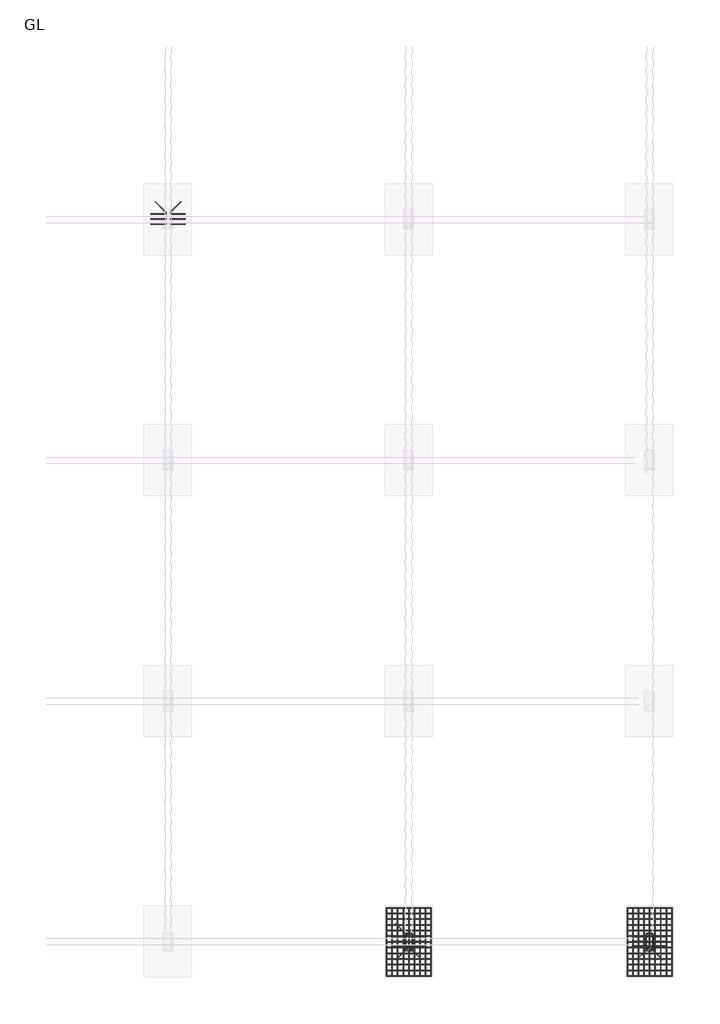
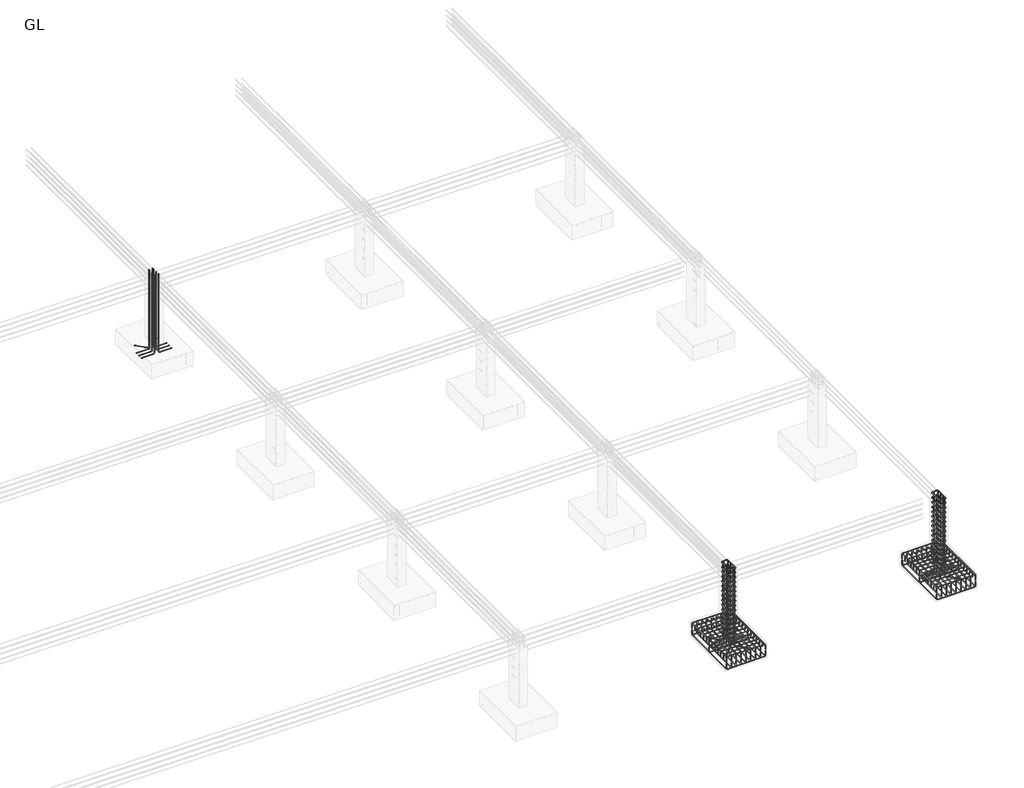
# One storey, part 10 of 16: 23 reinforcing bars.
"""IFC4 building model written with IfcOpenShell, lengths in millimetres."""

from ifc_helpers import new_model, si_unit, point, frame, origin, place, context, project, spatial, polyline, circle_curve, trimmed, segment, composite_curve, source, transform, mapped, element, save
from ifc_brep_helpers import swept_disk

model = new_model("IFC4")

# Units and contexts
model_context = context("Model", 3, world=origin())
ifc_project = project(units=[si_unit("LENGTHUNIT", "METRE", prefix="MILLI")], contexts=[model_context])

# Site, building, storey
site = spatial("IfcSite", under=ifc_project)
building = spatial("IfcBuilding", under=site)
storey = spatial("IfcBuildingStorey", under=building, Name="GL", Elevation=-1829.0)

# Reinforcing bars
placement = place(None, origin())
reinforcing_bar_shape = source(origin(), model_context, "Body", "SolidModel", [
    swept_disk(composite_curve([segment(polyline([(2141.0455621, -19415.1167521, -2089.0), (2141.0455621, -19415.1167521, -2213.0)]), True, "CONTINUOUS"), segment(trimmed(circle_curve(frame((2111.0455621, -19415.1167521, -2213.0), z_axis=(0.0, 1.0, 0.0), x_axis=(30.0, 0.0, 0.0)), 30.0), [point((2141.0455621, -19415.1167521, -2213.0))], [point((2111.0455621, -19415.1167521, -2243.0))], True, "CARTESIAN"), True, "CONTINUOUS"), segment(polyline([(2111.0455621, -19415.1167521, -2243.0), (1043.0455621, -19415.1167521, -2243.0)]), True, "CONTINUOUS"), segment(trimmed(circle_curve(frame((1043.0455621, -19415.1167521, -2213.0), z_axis=(0.0, 1.0, 0.0), x_axis=(0.0, 0.0, -30.0)), 30.0), [point((1043.0455621, -19415.1167521, -2243.0))], [point((1013.0455621, -19415.1167521, -2213.0))], True, "CARTESIAN"), True, "CONTINUOUS"), segment(polyline([(1013.0455621, -19415.1167521, -2213.0), (1013.0455621, -19415.1167521, -2089.0)]), True, "CONTINUOUS")], self_intersect=False), 6.0),
])
element("IfcReinforcingBar", 1, at=placement, inside=storey, context=model_context, shape_type="MappedRepresentation", body=[
    mapped(reinforcing_bar_shape, transform((0.0, 0.0, 0.0), x_axis=(1.0, 0.0, 0.0), y_axis=(0.0, 1.0, 0.0), z_axis=(0.0, 0.0, 1.0))),
    mapped(reinforcing_bar_shape, transform((0.0, -864.0, 0.0), x_axis=(1.0, 0.0, 0.0), y_axis=(0.0, 1.0, 0.0), z_axis=(0.0, 0.0, 1.0))),
    mapped(reinforcing_bar_shape, transform((0.0, -1728.0, 0.0), x_axis=(1.0, 0.0, 0.0), y_axis=(0.0, 1.0, 0.0), z_axis=(0.0, 0.0, 1.0))),
])
reinforcing_bar_2_shape = source(origin(), model_context, "Body", "SolidModel", [
    swept_disk(composite_curve([segment(polyline([(1013.0455621, -19415.1167521, -2022.436678), (1013.0455621, -19415.1167521, -1898.436678)]), True, "CONTINUOUS"), segment(trimmed(circle_curve(frame((1043.0455621, -19415.1167521, -1898.436678), z_axis=(0.0, 1.0, 0.0), x_axis=(-30.000000000000114, 0.0, 0.0)), 30.0), [point((1013.0455621, -19415.1167521, -1898.436678))], [point((1043.0455621, -19415.1167521, -1868.436678))], True, "CARTESIAN"), True, "CONTINUOUS"), segment(polyline([(1043.0455621, -19415.1167521, -1868.436678), (2111.0455621, -19415.1167521, -1868.436678)]), True, "CONTINUOUS"), segment(trimmed(circle_curve(frame((2111.0455621, -19415.1167521, -1898.436678), z_axis=(0.0, 1.0, 0.0), x_axis=(0.0, 0.0, 30.0)), 30.0), [point((2111.0455621, -19415.1167521, -1868.436678))], [point((2141.0455621, -19415.1167521, -1898.436678))], True, "CARTESIAN"), True, "CONTINUOUS"), segment(polyline([(2141.0455621, -19415.1167521, -1898.436678), (2141.0455621, -19415.1167521, -2022.436678)]), True, "CONTINUOUS")], self_intersect=False), 6.0),
])
element("IfcReinforcingBar", 2, at=placement, inside=storey, context=model_context, shape_type="MappedRepresentation", body=[
    mapped(reinforcing_bar_2_shape, transform((0.0, 0.0, 0.0), x_axis=(1.0, 0.0, 0.0), y_axis=(0.0, 1.0, 0.0), z_axis=(0.0, 0.0, 1.0))),
    mapped(reinforcing_bar_2_shape, transform((0.0, -144.0, 0.0), x_axis=(1.0, 0.0, 0.0), y_axis=(0.0, 1.0, 0.0), z_axis=(0.0, 0.0, 1.0))),
    mapped(reinforcing_bar_2_shape, transform((0.0, -288.0, 0.0), x_axis=(1.0, 0.0, 0.0), y_axis=(0.0, 1.0, 0.0), z_axis=(0.0, 0.0, 1.0))),
    mapped(reinforcing_bar_2_shape, transform((0.0, -432.0, 0.0), x_axis=(1.0, 0.0, 0.0), y_axis=(0.0, 1.0, 0.0), z_axis=(0.0, 0.0, 1.0))),
    mapped(reinforcing_bar_2_shape, transform((0.0, -576.0, 0.0), x_axis=(1.0, 0.0, 0.0), y_axis=(0.0, 1.0, 0.0), z_axis=(0.0, 0.0, 1.0))),
    mapped(reinforcing_bar_2_shape, transform((0.0, -720.0, 0.0), x_axis=(1.0, 0.0, 0.0), y_axis=(0.0, 1.0, 0.0), z_axis=(0.0, 0.0, 1.0))),
    mapped(reinforcing_bar_2_shape, transform((0.0, -864.0, 0.0), x_axis=(1.0, 0.0, 0.0), y_axis=(0.0, 1.0, 0.0), z_axis=(0.0, 0.0, 1.0))),
    mapped(reinforcing_bar_2_shape, transform((0.0, -1008.0, 0.0), x_axis=(1.0, 0.0, 0.0), y_axis=(0.0, 1.0, 0.0), z_axis=(0.0, 0.0, 1.0))),
    mapped(reinforcing_bar_2_shape, transform((0.0, -1152.0, 0.0), x_axis=(1.0, 0.0, 0.0), y_axis=(0.0, 1.0, 0.0), z_axis=(0.0, 0.0, 1.0))),
    mapped(reinforcing_bar_2_shape, transform((0.0, -1296.0, 0.0), x_axis=(1.0, 0.0, 0.0), y_axis=(0.0, 1.0, 0.0), z_axis=(0.0, 0.0, 1.0))),
    mapped(reinforcing_bar_2_shape, transform((0.0, -1440.0, 0.0), x_axis=(1.0, 0.0, 0.0), y_axis=(0.0, 1.0, 0.0), z_axis=(0.0, 0.0, 1.0))),
    mapped(reinforcing_bar_2_shape, transform((0.0, -1584.0, 0.0), x_axis=(1.0, 0.0, 0.0), y_axis=(0.0, 1.0, 0.0), z_axis=(0.0, 0.0, 1.0))),
    mapped(reinforcing_bar_2_shape, transform((0.0, -1728.0, 0.0), x_axis=(1.0, 0.0, 0.0), y_axis=(0.0, 1.0, 0.0), z_axis=(0.0, 0.0, 1.0))),
])
reinforcing_bar_3_shape = source(origin(), model_context, "Body", "SolidModel", [
    swept_disk(composite_curve([segment(polyline([(1013.0455621, -21143.1167521, -2027.5081232), (1013.0455621, -21143.1167521, -1903.5081232)]), True, "CONTINUOUS"), segment(trimmed(circle_curve(frame((1013.0455621, -21113.1167521, -1903.5081232), z_axis=(-1.0, 0.0, 0.0), x_axis=(0.0, -30.0, 0.0)), 30.0), [point((1013.0455621, -21143.1167521, -1903.5081232))], [point((1013.0455621, -21113.1167521, -1873.5081232))], True, "CARTESIAN"), True, "CONTINUOUS"), segment(polyline([(1013.0455621, -21113.1167521, -1873.5081232), (1013.0455621, -19445.1167521, -1873.5081232)]), True, "CONTINUOUS"), segment(trimmed(circle_curve(frame((1013.0455621, -19445.1167521, -1903.5081232), z_axis=(-1.0, 0.0, 0.0), x_axis=(0.0, 0.0, 30.0)), 30.0), [point((1013.0455621, -19445.1167521, -1873.5081232))], [point((1013.0455621, -19415.1167521, -1903.5081232))], True, "CARTESIAN"), True, "CONTINUOUS"), segment(polyline([(1013.0455621, -19415.1167521, -1903.5081232), (1013.0455621, -19415.1167521, -2027.5081232)]), True, "CONTINUOUS")], self_intersect=False), 6.0),
])
element("IfcReinforcingBar", 3, at=placement, inside=storey, context=model_context, shape_type="MappedRepresentation", body=[
    mapped(reinforcing_bar_3_shape, transform((0.0, 0.0, 0.0), x_axis=(1.0, 0.0, 0.0), y_axis=(0.0, 1.0, 0.0), z_axis=(0.0, 0.0, 1.0))),
    mapped(reinforcing_bar_3_shape, transform((141.0, 0.0, 0.0), x_axis=(1.0, 0.0, 0.0), y_axis=(0.0, 1.0, 0.0), z_axis=(0.0, 0.0, 1.0))),
    mapped(reinforcing_bar_3_shape, transform((282.0, 0.0, 0.0), x_axis=(1.0, 0.0, 0.0), y_axis=(0.0, 1.0, 0.0), z_axis=(0.0, 0.0, 1.0))),
    mapped(reinforcing_bar_3_shape, transform((423.0, 0.0, 0.0), x_axis=(1.0, 0.0, 0.0), y_axis=(0.0, 1.0, 0.0), z_axis=(0.0, 0.0, 1.0))),
    mapped(reinforcing_bar_3_shape, transform((564.0, 0.0, 0.0), x_axis=(1.0, 0.0, 0.0), y_axis=(0.0, 1.0, 0.0), z_axis=(0.0, 0.0, 1.0))),
    mapped(reinforcing_bar_3_shape, transform((705.0, 0.0, 0.0), x_axis=(1.0, 0.0, 0.0), y_axis=(0.0, 1.0, 0.0), z_axis=(0.0, 0.0, 1.0))),
    mapped(reinforcing_bar_3_shape, transform((846.0, 0.0, 0.0), x_axis=(1.0, 0.0, 0.0), y_axis=(0.0, 1.0, 0.0), z_axis=(0.0, 0.0, 1.0))),
    mapped(reinforcing_bar_3_shape, transform((987.0, 0.0, 0.0), x_axis=(1.0, 0.0, 0.0), y_axis=(0.0, 1.0, 0.0), z_axis=(0.0, 0.0, 1.0))),
    mapped(reinforcing_bar_3_shape, transform((1128.0, 0.0, 0.0), x_axis=(1.0, 0.0, 0.0), y_axis=(0.0, 1.0, 0.0), z_axis=(0.0, 0.0, 1.0))),
])
reinforcing_bar_4_shape = source(origin(), model_context, "Body", "SolidModel", [
    swept_disk(composite_curve([segment(polyline([(2141.0455621, -21143.1167521, -2080.6239909), (2141.0455621, -21143.1167521, -2204.6239909)]), True, "CONTINUOUS"), segment(trimmed(circle_curve(frame((2141.0455621, -21113.1167521, -2204.6239909), z_axis=(1.0, 0.0, 0.0), x_axis=(0.0, -30.0, 0.0)), 30.0), [point((2141.0455621, -21143.1167521, -2204.6239909))], [point((2141.0455621, -21113.1167521, -2234.6239909))], True, "CARTESIAN"), True, "CONTINUOUS"), segment(polyline([(2141.0455621, -21113.1167521, -2234.6239909), (2141.0455621, -19458.1421892, -2234.6239909)]), True, "CONTINUOUS"), segment(trimmed(circle_curve(frame((2141.0455621, -19458.1421892, -2204.6239909), z_axis=(1.0, 0.0, 0.0), x_axis=(0.0, 0.0, -30.0)), 30.0), [point((2141.0455621, -19458.1421892, -2234.6239909))], [point((2141.0455621, -19428.1421892, -2204.6239909))], True, "CARTESIAN"), True, "CONTINUOUS"), segment(polyline([(2141.0455621, -19428.1421892, -2204.6239909), (2141.0455621, -19428.1421892, -2080.6239909)]), True, "CONTINUOUS")], self_intersect=False), 6.0),
])
element("IfcReinforcingBar", 4, at=placement, inside=storey, context=model_context, shape_type="MappedRepresentation", body=[
    mapped(reinforcing_bar_4_shape, transform((0.0, 0.0, 0.0), x_axis=(1.0, 0.0, 0.0), y_axis=(0.0, 1.0, 0.0), z_axis=(0.0, 0.0, 1.0))),
    mapped(reinforcing_bar_4_shape, transform((-141.0, 0.0, 0.0), x_axis=(1.0, 0.0, 0.0), y_axis=(0.0, 1.0, 0.0), z_axis=(0.0, 0.0, 1.0))),
    mapped(reinforcing_bar_4_shape, transform((-282.0, 0.0, 0.0), x_axis=(1.0, 0.0, 0.0), y_axis=(0.0, 1.0, 0.0), z_axis=(0.0, 0.0, 1.0))),
    mapped(reinforcing_bar_4_shape, transform((-423.0, 0.0, 0.0), x_axis=(1.0, 0.0, 0.0), y_axis=(0.0, 1.0, 0.0), z_axis=(0.0, 0.0, 1.0))),
    mapped(reinforcing_bar_4_shape, transform((-564.0, 0.0, 0.0), x_axis=(1.0, 0.0, 0.0), y_axis=(0.0, 1.0, 0.0), z_axis=(0.0, 0.0, 1.0))),
    mapped(reinforcing_bar_4_shape, transform((-705.0, 0.0, 0.0), x_axis=(1.0, 0.0, 0.0), y_axis=(0.0, 1.0, 0.0), z_axis=(0.0, 0.0, 1.0))),
    mapped(reinforcing_bar_4_shape, transform((-846.0, 0.0, 0.0), x_axis=(1.0, 0.0, 0.0), y_axis=(0.0, 1.0, 0.0), z_axis=(0.0, 0.0, 1.0))),
    mapped(reinforcing_bar_4_shape, transform((-987.0, 0.0, 0.0), x_axis=(1.0, 0.0, 0.0), y_axis=(0.0, 1.0, 0.0), z_axis=(0.0, 0.0, 1.0))),
    mapped(reinforcing_bar_4_shape, transform((-1128.0, 0.0, 0.0), x_axis=(1.0, 0.0, 0.0), y_axis=(0.0, 1.0, 0.0), z_axis=(0.0, 0.0, 1.0))),
])
reinforcing_bar_5_shape = source(origin(), model_context, "Body", "SolidModel", [
    swept_disk(composite_curve([segment(polyline([(8237.0455621, -19415.1167521, -2089.0), (8237.0455621, -19415.1167521, -2213.0)]), True, "CONTINUOUS"), segment(trimmed(circle_curve(frame((8207.0455621, -19415.1167521, -2213.0), z_axis=(0.0, 1.0, 0.0), x_axis=(30.0, 0.0, 0.0)), 30.0), [point((8237.0455621, -19415.1167521, -2213.0))], [point((8207.0455621, -19415.1167521, -2243.0))], True, "CARTESIAN"), True, "CONTINUOUS"), segment(polyline([(8207.0455621, -19415.1167521, -2243.0), (7139.0455621, -19415.1167521, -2243.0)]), True, "CONTINUOUS"), segment(trimmed(circle_curve(frame((7139.0455621, -19415.1167521, -2213.0), z_axis=(0.0, 1.0, 0.0), x_axis=(0.0, 0.0, -30.0)), 30.0), [point((7139.0455621, -19415.1167521, -2243.0))], [point((7109.0455621, -19415.1167521, -2213.0))], True, "CARTESIAN"), True, "CONTINUOUS"), segment(polyline([(7109.0455621, -19415.1167521, -2213.0), (7109.0455621, -19415.1167521, -2089.0)]), True, "CONTINUOUS")], self_intersect=False), 6.0),
])
element("IfcReinforcingBar", 5, at=placement, inside=storey, context=model_context, shape_type="MappedRepresentation", body=[
    mapped(reinforcing_bar_5_shape, transform((0.0, 0.0, 0.0), x_axis=(1.0, 0.0, 0.0), y_axis=(0.0, 1.0, 0.0), z_axis=(0.0, 0.0, 1.0))),
    mapped(reinforcing_bar_5_shape, transform((0.0, -864.0, 0.0), x_axis=(1.0, 0.0, 0.0), y_axis=(0.0, 1.0, 0.0), z_axis=(0.0, 0.0, 1.0))),
    mapped(reinforcing_bar_5_shape, transform((0.0, -1728.0, 0.0), x_axis=(1.0, 0.0, 0.0), y_axis=(0.0, 1.0, 0.0), z_axis=(0.0, 0.0, 1.0))),
])
reinforcing_bar_6_shape = source(origin(), model_context, "Body", "SolidModel", [
    swept_disk(composite_curve([segment(polyline([(7109.0455621, -19415.1167521, -2022.436678), (7109.0455621, -19415.1167521, -1898.436678)]), True, "CONTINUOUS"), segment(trimmed(circle_curve(frame((7139.0455621, -19415.1167521, -1898.436678), z_axis=(0.0, 1.0, 0.0), x_axis=(-30.0, 0.0, 0.0)), 30.0), [point((7109.0455621, -19415.1167521, -1898.436678))], [point((7139.0455621, -19415.1167521, -1868.436678))], True, "CARTESIAN"), True, "CONTINUOUS"), segment(polyline([(7139.0455621, -19415.1167521, -1868.436678), (8207.0455621, -19415.1167521, -1868.436678)]), True, "CONTINUOUS"), segment(trimmed(circle_curve(frame((8207.0455621, -19415.1167521, -1898.436678), z_axis=(0.0, 1.0, 0.0), x_axis=(0.0, 0.0, 30.0)), 30.0), [point((8207.0455621, -19415.1167521, -1868.436678))], [point((8237.0455621, -19415.1167521, -1898.436678))], True, "CARTESIAN"), True, "CONTINUOUS"), segment(polyline([(8237.0455621, -19415.1167521, -1898.436678), (8237.0455621, -19415.1167521, -2022.436678)]), True, "CONTINUOUS")], self_intersect=False), 6.0),
])
element("IfcReinforcingBar", 6, at=placement, inside=storey, context=model_context, shape_type="MappedRepresentation", body=[
    mapped(reinforcing_bar_6_shape, transform((0.0, 0.0, 0.0), x_axis=(1.0, 0.0, 0.0), y_axis=(0.0, 1.0, 0.0), z_axis=(0.0, 0.0, 1.0))),
    mapped(reinforcing_bar_6_shape, transform((0.0, -144.0, 0.0), x_axis=(1.0, 0.0, 0.0), y_axis=(0.0, 1.0, 0.0), z_axis=(0.0, 0.0, 1.0))),
    mapped(reinforcing_bar_6_shape, transform((0.0, -288.0, 0.0), x_axis=(1.0, 0.0, 0.0), y_axis=(0.0, 1.0, 0.0), z_axis=(0.0, 0.0, 1.0))),
    mapped(reinforcing_bar_6_shape, transform((0.0, -432.0, 0.0), x_axis=(1.0, 0.0, 0.0), y_axis=(0.0, 1.0, 0.0), z_axis=(0.0, 0.0, 1.0))),
    mapped(reinforcing_bar_6_shape, transform((0.0, -576.0, 0.0), x_axis=(1.0, 0.0, 0.0), y_axis=(0.0, 1.0, 0.0), z_axis=(0.0, 0.0, 1.0))),
    mapped(reinforcing_bar_6_shape, transform((0.0, -720.0, 0.0), x_axis=(1.0, 0.0, 0.0), y_axis=(0.0, 1.0, 0.0), z_axis=(0.0, 0.0, 1.0))),
    mapped(reinforcing_bar_6_shape, transform((0.0, -864.0, 0.0), x_axis=(1.0, 0.0, 0.0), y_axis=(0.0, 1.0, 0.0), z_axis=(0.0, 0.0, 1.0))),
    mapped(reinforcing_bar_6_shape, transform((0.0, -1008.0, 0.0), x_axis=(1.0, 0.0, 0.0), y_axis=(0.0, 1.0, 0.0), z_axis=(0.0, 0.0, 1.0))),
    mapped(reinforcing_bar_6_shape, transform((0.0, -1152.0, 0.0), x_axis=(1.0, 0.0, 0.0), y_axis=(0.0, 1.0, 0.0), z_axis=(0.0, 0.0, 1.0))),
    mapped(reinforcing_bar_6_shape, transform((0.0, -1296.0, 0.0), x_axis=(1.0, 0.0, 0.0), y_axis=(0.0, 1.0, 0.0), z_axis=(0.0, 0.0, 1.0))),
    mapped(reinforcing_bar_6_shape, transform((0.0, -1440.0, 0.0), x_axis=(1.0, 0.0, 0.0), y_axis=(0.0, 1.0, 0.0), z_axis=(0.0, 0.0, 1.0))),
    mapped(reinforcing_bar_6_shape, transform((0.0, -1584.0, 0.0), x_axis=(1.0, 0.0, 0.0), y_axis=(0.0, 1.0, 0.0), z_axis=(0.0, 0.0, 1.0))),
    mapped(reinforcing_bar_6_shape, transform((0.0, -1728.0, 0.0), x_axis=(1.0, 0.0, 0.0), y_axis=(0.0, 1.0, 0.0), z_axis=(0.0, 0.0, 1.0))),
])
reinforcing_bar_7_shape = source(origin(), model_context, "Body", "SolidModel", [
    swept_disk(composite_curve([segment(polyline([(7109.0455621, -21143.1167521, -2027.5081232), (7109.0455621, -21143.1167521, -1903.5081232)]), True, "CONTINUOUS"), segment(trimmed(circle_curve(frame((7109.0455621, -21113.1167521, -1903.5081232), z_axis=(-1.0, 0.0, 0.0), x_axis=(0.0, -30.0, 0.0)), 30.0), [point((7109.0455621, -21143.1167521, -1903.5081232))], [point((7109.0455621, -21113.1167521, -1873.5081232))], True, "CARTESIAN"), True, "CONTINUOUS"), segment(polyline([(7109.0455621, -21113.1167521, -1873.5081232), (7109.0455621, -19445.1167521, -1873.5081232)]), True, "CONTINUOUS"), segment(trimmed(circle_curve(frame((7109.0455621, -19445.1167521, -1903.5081232), z_axis=(-1.0, 0.0, 0.0), x_axis=(0.0, 0.0, 30.0)), 30.0), [point((7109.0455621, -19445.1167521, -1873.5081232))], [point((7109.0455621, -19415.1167521, -1903.5081232))], True, "CARTESIAN"), True, "CONTINUOUS"), segment(polyline([(7109.0455621, -19415.1167521, -1903.5081232), (7109.0455621, -19415.1167521, -2027.5081232)]), True, "CONTINUOUS")], self_intersect=False), 6.0),
])
element("IfcReinforcingBar", 7, at=placement, inside=storey, context=model_context, shape_type="MappedRepresentation", body=[
    mapped(reinforcing_bar_7_shape, transform((0.0, 0.0, 0.0), x_axis=(1.0, 0.0, 0.0), y_axis=(0.0, 1.0, 0.0), z_axis=(0.0, 0.0, 1.0))),
    mapped(reinforcing_bar_7_shape, transform((141.0, 0.0, 0.0), x_axis=(1.0, 0.0, 0.0), y_axis=(0.0, 1.0, 0.0), z_axis=(0.0, 0.0, 1.0))),
    mapped(reinforcing_bar_7_shape, transform((282.0, 0.0, 0.0), x_axis=(1.0, 0.0, 0.0), y_axis=(0.0, 1.0, 0.0), z_axis=(0.0, 0.0, 1.0))),
    mapped(reinforcing_bar_7_shape, transform((423.0, 0.0, 0.0), x_axis=(1.0, 0.0, 0.0), y_axis=(0.0, 1.0, 0.0), z_axis=(0.0, 0.0, 1.0))),
    mapped(reinforcing_bar_7_shape, transform((564.0, 0.0, 0.0), x_axis=(1.0, 0.0, 0.0), y_axis=(0.0, 1.0, 0.0), z_axis=(0.0, 0.0, 1.0))),
    mapped(reinforcing_bar_7_shape, transform((705.0, 0.0, 0.0), x_axis=(1.0, 0.0, 0.0), y_axis=(0.0, 1.0, 0.0), z_axis=(0.0, 0.0, 1.0))),
    mapped(reinforcing_bar_7_shape, transform((846.0, 0.0, 0.0), x_axis=(1.0, 0.0, 0.0), y_axis=(0.0, 1.0, 0.0), z_axis=(0.0, 0.0, 1.0))),
    mapped(reinforcing_bar_7_shape, transform((987.0, 0.0, 0.0), x_axis=(1.0, 0.0, 0.0), y_axis=(0.0, 1.0, 0.0), z_axis=(0.0, 0.0, 1.0))),
    mapped(reinforcing_bar_7_shape, transform((1128.0, 0.0, 0.0), x_axis=(1.0, 0.0, 0.0), y_axis=(0.0, 1.0, 0.0), z_axis=(0.0, 0.0, 1.0))),
])
reinforcing_bar_8_shape = source(origin(), model_context, "Body", "SolidModel", [
    swept_disk(composite_curve([segment(polyline([(8237.0455621, -21143.1167521, -2080.6239909), (8237.0455621, -21143.1167521, -2204.6239909)]), True, "CONTINUOUS"), segment(trimmed(circle_curve(frame((8237.0455621, -21113.1167521, -2204.6239909), z_axis=(1.0, 0.0, 0.0), x_axis=(0.0, -30.0, 0.0)), 30.0), [point((8237.0455621, -21143.1167521, -2204.6239909))], [point((8237.0455621, -21113.1167521, -2234.6239909))], True, "CARTESIAN"), True, "CONTINUOUS"), segment(polyline([(8237.0455621, -21113.1167521, -2234.6239909), (8237.0455621, -19458.1421892, -2234.6239909)]), True, "CONTINUOUS"), segment(trimmed(circle_curve(frame((8237.0455621, -19458.1421892, -2204.6239909), z_axis=(1.0, 0.0, 0.0), x_axis=(0.0, 0.0, -30.0)), 30.0), [point((8237.0455621, -19458.1421892, -2234.6239909))], [point((8237.0455621, -19428.1421892, -2204.6239909))], True, "CARTESIAN"), True, "CONTINUOUS"), segment(polyline([(8237.0455621, -19428.1421892, -2204.6239909), (8237.0455621, -19428.1421892, -2080.6239909)]), True, "CONTINUOUS")], self_intersect=False), 6.0),
])
element("IfcReinforcingBar", 8, at=placement, inside=storey, context=model_context, shape_type="MappedRepresentation", body=[
    mapped(reinforcing_bar_8_shape, transform((0.0, 0.0, 0.0), x_axis=(1.0, 0.0, 0.0), y_axis=(0.0, 1.0, 0.0), z_axis=(0.0, 0.0, 1.0))),
    mapped(reinforcing_bar_8_shape, transform((-141.0, 0.0, 0.0), x_axis=(1.0, 0.0, 0.0), y_axis=(0.0, 1.0, 0.0), z_axis=(0.0, 0.0, 1.0))),
    mapped(reinforcing_bar_8_shape, transform((-282.0, 0.0, 0.0), x_axis=(1.0, 0.0, 0.0), y_axis=(0.0, 1.0, 0.0), z_axis=(0.0, 0.0, 1.0))),
    mapped(reinforcing_bar_8_shape, transform((-423.0, 0.0, 0.0), x_axis=(1.0, 0.0, 0.0), y_axis=(0.0, 1.0, 0.0), z_axis=(0.0, 0.0, 1.0))),
    mapped(reinforcing_bar_8_shape, transform((-564.0, 0.0, 0.0), x_axis=(1.0, 0.0, 0.0), y_axis=(0.0, 1.0, 0.0), z_axis=(0.0, 0.0, 1.0))),
    mapped(reinforcing_bar_8_shape, transform((-705.0, 0.0, 0.0), x_axis=(1.0, 0.0, 0.0), y_axis=(0.0, 1.0, 0.0), z_axis=(0.0, 0.0, 1.0))),
    mapped(reinforcing_bar_8_shape, transform((-846.0, 0.0, 0.0), x_axis=(1.0, 0.0, 0.0), y_axis=(0.0, 1.0, 0.0), z_axis=(0.0, 0.0, 1.0))),
    mapped(reinforcing_bar_8_shape, transform((-987.0, 0.0, 0.0), x_axis=(1.0, 0.0, 0.0), y_axis=(0.0, 1.0, 0.0), z_axis=(0.0, 0.0, 1.0))),
    mapped(reinforcing_bar_8_shape, transform((-1128.0, 0.0, 0.0), x_axis=(1.0, 0.0, 0.0), y_axis=(0.0, 1.0, 0.0), z_axis=(0.0, 0.0, 1.0))),
])
element("IfcReinforcingBar", 9, at=placement, inside=storey, context=model_context, shape_type="SolidModel", body=[
    swept_disk(composite_curve([segment(polyline([(-4576.0642232, -1806.1692603, 241.0), (-4576.0642232, -1806.1692603, -2129.0)]), True, "CONTINUOUS"), segment(trimmed(circle_curve(frame((-4597.2774266, -1784.9560568, -2129.0), z_axis=(0.7071067811865218, 0.7071067811865733, 0.0), x_axis=(21.213203399999657, -21.213203499999963, 0.0)), 30.0), [point((-4576.0642232, -1806.1692603, -2129.0))], [point((-4597.2774266, -1784.9560568, -2159.0))], True, "CARTESIAN"), True, "CONTINUOUS"), segment(polyline([(-4597.2774266, -1784.9560568, -2159.0), (-4844.7648, -1537.4686834, -2159.0)]), True, "CONTINUOUS")], self_intersect=False), 6.0),
])
element("IfcReinforcingBar", 10, at=placement, inside=storey, context=model_context, shape_type="SolidModel", body=[
    swept_disk(composite_curve([segment(polyline([(-4461.8446527, -1806.1692603, 241.0), (-4461.8446527, -1806.1692603, -2129.0)]), True, "CONTINUOUS"), segment(trimmed(circle_curve(frame((-4440.6314492, -1784.9560568, -2129.0), z_axis=(0.7071067811865157, -0.7071067811865794, 0.0), x_axis=(-21.21320349999951, -21.213203499999963, 0.0)), 30.0), [point((-4461.8446527, -1806.1692603, -2129.0))], [point((-4440.6314492, -1784.9560568, -2159.0))], True, "CARTESIAN"), True, "CONTINUOUS"), segment(polyline([(-4440.6314492, -1784.9560568, -2159.0), (-4193.1440758, -1537.4686834, -2159.0)]), True, "CONTINUOUS")], self_intersect=False), 6.0),
])
reinforcing_bar_9_shape = source(origin(), model_context, "Body", "SolidModel", [
    swept_disk(composite_curve([segment(polyline([(-4576.0642232, -2098.9117405, 241.0), (-4576.0642232, -2098.9117405, -2129.0)]), True, "CONTINUOUS"), segment(trimmed(circle_curve(frame((-4606.0642232, -2098.9117405, -2129.0), z_axis=(0.0, 1.0, 0.0), x_axis=(30.0, 0.0, 0.0)), 30.0), [point((-4576.0642232, -2098.9117405, -2129.0))], [point((-4606.0642232, -2098.9117405, -2159.0))], True, "CARTESIAN"), True, "CONTINUOUS"), segment(polyline([(-4606.0642232, -2098.9117405, -2159.0), (-4956.0642232, -2098.9117405, -2159.0)]), True, "CONTINUOUS")], self_intersect=False), 6.0),
])
element("IfcReinforcingBar", 11, at=placement, inside=storey, context=model_context, shape_type="MappedRepresentation", body=[
    mapped(reinforcing_bar_9_shape, transform((0.0, 0.0, 0.0), x_axis=(1.0, 0.0, 0.0), y_axis=(0.0, 1.0, 0.0), z_axis=(0.0, 0.0, 1.0))),
    mapped(reinforcing_bar_9_shape, transform((0.0, 123.5823926, 0.0), x_axis=(1.0, 0.0, 0.0), y_axis=(0.0, 1.0, 0.0), z_axis=(0.0, 0.0, 1.0))),
    mapped(reinforcing_bar_9_shape, transform((0.0, 247.1647853, 0.0), x_axis=(1.0, 0.0, 0.0), y_axis=(0.0, 1.0, 0.0), z_axis=(0.0, 0.0, 1.0))),
])
reinforcing_bar_10_shape = source(origin(), model_context, "Body", "SolidModel", [
    swept_disk(composite_curve([segment(polyline([(-4461.8446527, -2098.9117405, 241.0), (-4461.8446527, -2098.9117405, -2129.0)]), True, "CONTINUOUS"), segment(trimmed(circle_curve(frame((-4431.8446527, -2098.9117405, -2129.0), z_axis=(0.0, -1.0, 0.0), x_axis=(-30.0, 0.0, 0.0)), 30.0), [point((-4461.8446527, -2098.9117405, -2129.0))], [point((-4431.8446527, -2098.9117405, -2159.0))], True, "CARTESIAN"), True, "CONTINUOUS"), segment(polyline([(-4431.8446527, -2098.9117405, -2159.0), (-4081.8446527, -2098.9117405, -2159.0)]), True, "CONTINUOUS")], self_intersect=False), 6.0),
])
element("IfcReinforcingBar", 12, at=placement, inside=storey, context=model_context, shape_type="MappedRepresentation", body=[
    mapped(reinforcing_bar_10_shape, transform((0.0, 0.0, 0.0), x_axis=(1.0, 0.0, 0.0), y_axis=(0.0, 1.0, 0.0), z_axis=(0.0, 0.0, 1.0))),
    mapped(reinforcing_bar_10_shape, transform((0.0, 123.5823926, 0.0), x_axis=(1.0, 0.0, 0.0), y_axis=(0.0, 1.0, 0.0), z_axis=(0.0, 0.0, 1.0))),
    mapped(reinforcing_bar_10_shape, transform((0.0, 247.1647853, 0.0), x_axis=(1.0, 0.0, 0.0), y_axis=(0.0, 1.0, 0.0), z_axis=(0.0, 0.0, 1.0))),
])
reinforcing_bar_11_shape = source(origin(), model_context, "Body", "SolidModel", [
    swept_disk(composite_curve([segment(polyline([(7680.5135995, -20354.2223078, -1793.0), (7592.8323586, -20441.9035486, -1793.0)]), True, "CONTINUOUS"), segment(trimmed(circle_curve(frame((7614.0455621, -20463.1167521, -1793.0), z_axis=(0.0, 0.0, 1.0), x_axis=(-21.213203500000418, 21.21320349999951, 0.0)), 30.0), [point((7592.8323586, -20441.9035486, -1793.0))], [point((7614.0455621, -20493.1167521, -1793.0))], True, "CARTESIAN"), True, "CONTINUOUS"), segment(polyline([(7614.0455621, -20493.1167521, -1793.0), (7732.0455621, -20493.1167521, -1793.0)]), True, "CONTINUOUS"), segment(trimmed(circle_curve(frame((7732.0455621, -20463.1167521, -1793.0), z_axis=(0.0, 0.0, 1.0), x_axis=(0.0, -30.0, 0.0)), 30.0), [point((7732.0455621, -20493.1167521, -1793.0))], [point((7762.0455621, -20463.1167521, -1793.0))], True, "CARTESIAN"), True, "CONTINUOUS"), segment(polyline([(7762.0455621, -20463.1167521, -1793.0), (7762.0455621, -20095.1167521, -1793.0)]), True, "CONTINUOUS"), segment(trimmed(circle_curve(frame((7732.1135038, -20095.1167521, -1795.0178916), z_axis=(-0.06726305234213417, 0.0, 0.9977352764083365), x_axis=(29.93205829999988, 0.0, 2.0178915999999845)), 30.0), [point((7762.0455621, -20095.1167521, -1793.0))], [point((7732.1135038, -20065.1167521, -1795.0178916))], True, "CARTESIAN"), True, "CONTINUOUS"), segment(polyline([(7732.1135038, -20065.1167521, -1795.0178916), (7613.9776204, -20065.1167521, -1802.9821084)]), True, "CONTINUOUS"), segment(trimmed(circle_curve(frame((7613.9776204, -20095.1167521, -1802.9821084), z_axis=(-0.06726305234213417, 0.0, 0.9977352764083365), x_axis=(0.0, 30.0, 0.0)), 30.0), [point((7613.9776204, -20065.1167521, -1802.9821084))], [point((7584.0455621, -20095.1167521, -1805.0))], True, "CARTESIAN"), True, "CONTINUOUS"), segment(polyline([(7584.0455621, -20095.1167521, -1805.0), (7584.0455621, -20463.1167521, -1805.0)]), True, "CONTINUOUS"), segment(trimmed(circle_curve(frame((7614.0455621, -20463.1167521, -1805.0), z_axis=(0.0, 0.0, 1.0), x_axis=(-30.0, 0.0, 0.0)), 30.0), [point((7584.0455621, -20463.1167521, -1805.0))], [point((7635.2587655, -20484.3299555, -1805.0))], True, "CARTESIAN"), True, "CONTINUOUS"), segment(polyline([(7635.2587655, -20484.3299555, -1805.0), (7722.9400064, -20396.6487146, -1805.0)]), True, "CONTINUOUS")], self_intersect=False), 6.0),
])
element("IfcReinforcingBar", 13, at=placement, inside=storey, context=model_context, shape_type="MappedRepresentation", body=[
    mapped(reinforcing_bar_11_shape, transform((0.0, 0.0, 0.0), x_axis=(1.0, 0.0, 0.0), y_axis=(0.0, 1.0, 0.0), z_axis=(0.0, 0.0, 1.0))),
    mapped(reinforcing_bar_11_shape, transform((0.0, 0.0, 144.8571429), x_axis=(1.0, 0.0, 0.0), y_axis=(0.0, 1.0, 0.0), z_axis=(0.0, 0.0, 1.0))),
    mapped(reinforcing_bar_11_shape, transform((0.0, 0.0, 289.7142857), x_axis=(1.0, 0.0, 0.0), y_axis=(0.0, 1.0, 0.0), z_axis=(0.0, 0.0, 1.0))),
    mapped(reinforcing_bar_11_shape, transform((0.0, 0.0, 434.5714286), x_axis=(1.0, 0.0, 0.0), y_axis=(0.0, 1.0, 0.0), z_axis=(0.0, 0.0, 1.0))),
    mapped(reinforcing_bar_11_shape, transform((0.0, 0.0, 579.4285714), x_axis=(1.0, 0.0, 0.0), y_axis=(0.0, 1.0, 0.0), z_axis=(0.0, 0.0, 1.0))),
    mapped(reinforcing_bar_11_shape, transform((0.0, 0.0, 724.2857143), x_axis=(1.0, 0.0, 0.0), y_axis=(0.0, 1.0, 0.0), z_axis=(0.0, 0.0, 1.0))),
    mapped(reinforcing_bar_11_shape, transform((0.0, 0.0, 869.1428571), x_axis=(1.0, 0.0, 0.0), y_axis=(0.0, 1.0, 0.0), z_axis=(0.0, 0.0, 1.0))),
    mapped(reinforcing_bar_11_shape, transform((0.0, 0.0, 1014.0), x_axis=(1.0, 0.0, 0.0), y_axis=(0.0, 1.0, 0.0), z_axis=(0.0, 0.0, 1.0))),
    mapped(reinforcing_bar_11_shape, transform((0.0, 0.0, 1158.8571429), x_axis=(1.0, 0.0, 0.0), y_axis=(0.0, 1.0, 0.0), z_axis=(0.0, 0.0, 1.0))),
    mapped(reinforcing_bar_11_shape, transform((0.0, 0.0, 1303.7142857), x_axis=(1.0, 0.0, 0.0), y_axis=(0.0, 1.0, 0.0), z_axis=(0.0, 0.0, 1.0))),
    mapped(reinforcing_bar_11_shape, transform((0.0, 0.0, 1448.5714286), x_axis=(1.0, 0.0, 0.0), y_axis=(0.0, 1.0, 0.0), z_axis=(0.0, 0.0, 1.0))),
    mapped(reinforcing_bar_11_shape, transform((0.0, 0.0, 1593.4285714), x_axis=(1.0, 0.0, 0.0), y_axis=(0.0, 1.0, 0.0), z_axis=(0.0, 0.0, 1.0))),
    mapped(reinforcing_bar_11_shape, transform((0.0, 0.0, 1738.2857143), x_axis=(1.0, 0.0, 0.0), y_axis=(0.0, 1.0, 0.0), z_axis=(0.0, 0.0, 1.0))),
    mapped(reinforcing_bar_11_shape, transform((0.0, 0.0, 1883.1428571), x_axis=(1.0, 0.0, 0.0), y_axis=(0.0, 1.0, 0.0), z_axis=(0.0, 0.0, 1.0))),
    mapped(reinforcing_bar_11_shape, transform((0.0, 0.0, 2028.0), x_axis=(1.0, 0.0, 0.0), y_axis=(0.0, 1.0, 0.0), z_axis=(0.0, 0.0, 1.0))),
])
element("IfcReinforcingBar", 14, at=placement, inside=storey, context=model_context, shape_type="SolidModel", body=[
    swept_disk(composite_curve([segment(polyline([(7615.9357768, -20464.0642439, 241.0), (7615.9357768, -20464.0642439, -2129.0)]), True, "CONTINUOUS"), segment(trimmed(circle_curve(frame((7594.7225734, -20485.2774473, -2129.0), z_axis=(-0.7071067811865187, 0.7071067811865764, 0.0), x_axis=(21.213203399999657, 21.213203399998747, 0.0)), 30.0), [point((7615.9357768, -20464.0642439, -2129.0))], [point((7594.7225734, -20485.2774473, -2159.0))], True, "CARTESIAN"), True, "CONTINUOUS"), segment(polyline([(7594.7225734, -20485.2774473, -2159.0), (7347.2352, -20732.7648207, -2159.0)]), True, "CONTINUOUS")], self_intersect=False), 6.0),
])
element("IfcReinforcingBar", 15, at=placement, inside=storey, context=model_context, shape_type="SolidModel", body=[
    swept_disk(composite_curve([segment(polyline([(7730.1553473, -20464.0642439, 241.0), (7730.1553473, -20464.0642439, -2129.0)]), True, "CONTINUOUS"), segment(trimmed(circle_curve(frame((7751.3685508, -20485.2774473, -2129.0), z_axis=(-0.7071067811865248, -0.7071067811865703, 0.0), x_axis=(-21.21320349999951, 21.213203399998747, 0.0)), 30.0), [point((7730.1553473, -20464.0642439, -2129.0))], [point((7751.3685508, -20485.2774473, -2159.0))], True, "CARTESIAN"), True, "CONTINUOUS"), segment(polyline([(7751.3685508, -20485.2774473, -2159.0), (7998.8559242, -20732.7648207, -2159.0)]), True, "CONTINUOUS")], self_intersect=False), 6.0),
])
reinforcing_bar_12_shape = source(origin(), model_context, "Body", "SolidModel", [
    swept_disk(composite_curve([segment(polyline([(7615.9357768, -20386.9117405, 241.0), (7615.9357768, -20386.9117405, -2129.0)]), True, "CONTINUOUS"), segment(trimmed(circle_curve(frame((7585.9357768, -20386.9117405, -2129.0), z_axis=(0.0, 1.0, 0.0), x_axis=(30.0, 0.0, 0.0)), 30.0), [point((7615.9357768, -20386.9117405, -2129.0))], [point((7585.9357768, -20386.9117405, -2159.0))], True, "CARTESIAN"), True, "CONTINUOUS"), segment(polyline([(7585.9357768, -20386.9117405, -2159.0), (7235.9357768, -20386.9117405, -2159.0)]), True, "CONTINUOUS")], self_intersect=False), 6.0),
])
element("IfcReinforcingBar", 16, at=placement, inside=storey, context=model_context, shape_type="MappedRepresentation", body=[
    mapped(reinforcing_bar_12_shape, transform((0.0, 0.0, 0.0), x_axis=(1.0, 0.0, 0.0), y_axis=(0.0, 1.0, 0.0), z_axis=(0.0, 0.0, 1.0))),
    mapped(reinforcing_bar_12_shape, transform((0.0, 123.5823926, 0.0), x_axis=(1.0, 0.0, 0.0), y_axis=(0.0, 1.0, 0.0), z_axis=(0.0, 0.0, 1.0))),
    mapped(reinforcing_bar_12_shape, transform((0.0, 247.1647853, 0.0), x_axis=(1.0, 0.0, 0.0), y_axis=(0.0, 1.0, 0.0), z_axis=(0.0, 0.0, 1.0))),
])
reinforcing_bar_13_shape = source(origin(), model_context, "Body", "SolidModel", [
    swept_disk(composite_curve([segment(polyline([(7730.1553473, -20386.9117405, 241.0), (7730.1553473, -20386.9117405, -2129.0)]), True, "CONTINUOUS"), segment(trimmed(circle_curve(frame((7760.1553473, -20386.9117405, -2129.0), z_axis=(0.0, -1.0, 0.0), x_axis=(-30.0, 0.0, 0.0)), 30.0), [point((7730.1553473, -20386.9117405, -2129.0))], [point((7760.1553473, -20386.9117405, -2159.0))], True, "CARTESIAN"), True, "CONTINUOUS"), segment(polyline([(7760.1553473, -20386.9117405, -2159.0), (8110.1553473, -20386.9117405, -2159.0)]), True, "CONTINUOUS")], self_intersect=False), 6.0),
])
element("IfcReinforcingBar", 17, at=placement, inside=storey, context=model_context, shape_type="MappedRepresentation", body=[
    mapped(reinforcing_bar_13_shape, transform((0.0, 0.0, 0.0), x_axis=(1.0, 0.0, 0.0), y_axis=(0.0, 1.0, 0.0), z_axis=(0.0, 0.0, 1.0))),
    mapped(reinforcing_bar_13_shape, transform((0.0, 123.5823926, 0.0), x_axis=(1.0, 0.0, 0.0), y_axis=(0.0, 1.0, 0.0), z_axis=(0.0, 0.0, 1.0))),
    mapped(reinforcing_bar_13_shape, transform((0.0, 247.1647853, 0.0), x_axis=(1.0, 0.0, 0.0), y_axis=(0.0, 1.0, 0.0), z_axis=(0.0, 0.0, 1.0))),
])
reinforcing_bar_14_shape = source(origin(), model_context, "Body", "SolidModel", [
    swept_disk(composite_curve([segment(polyline([(1584.5135995, -20354.2223078, -1793.0), (1496.8323586, -20441.9035486, -1793.0)]), True, "CONTINUOUS"), segment(trimmed(circle_curve(frame((1518.0455621, -20463.1167521, -1793.0), z_axis=(0.0, 0.0, 1.0), x_axis=(-21.21320350000019, 21.21320349999951, 0.0)), 30.0), [point((1496.8323586, -20441.9035486, -1793.0))], [point((1518.0455621, -20493.1167521, -1793.0))], True, "CARTESIAN"), True, "CONTINUOUS"), segment(polyline([(1518.0455621, -20493.1167521, -1793.0), (1636.0455621, -20493.1167521, -1793.0)]), True, "CONTINUOUS"), segment(trimmed(circle_curve(frame((1636.0455621, -20463.1167521, -1793.0), z_axis=(0.0, 0.0, 1.0), x_axis=(0.0, -30.0, 0.0)), 30.0), [point((1636.0455621, -20493.1167521, -1793.0))], [point((1666.0455621, -20463.1167521, -1793.0))], True, "CARTESIAN"), True, "CONTINUOUS"), segment(polyline([(1666.0455621, -20463.1167521, -1793.0), (1666.0455621, -20095.1167521, -1793.0)]), True, "CONTINUOUS"), segment(trimmed(circle_curve(frame((1636.1135038, -20095.1167521, -1795.0178916), z_axis=(-0.06726305234213417, 0.0, 0.9977352764083365), x_axis=(29.932058300000108, 0.0, 2.0178915999999845)), 30.0), [point((1666.0455621, -20095.1167521, -1793.0))], [point((1636.1135038, -20065.1167521, -1795.0178916))], True, "CARTESIAN"), True, "CONTINUOUS"), segment(polyline([(1636.1135038, -20065.1167521, -1795.0178916), (1517.9776204, -20065.1167521, -1802.9821084)]), True, "CONTINUOUS"), segment(trimmed(circle_curve(frame((1517.9776204, -20095.1167521, -1802.9821084), z_axis=(-0.06726305234213417, 0.0, 0.9977352764083365), x_axis=(0.0, 30.0, 0.0)), 30.0), [point((1517.9776204, -20065.1167521, -1802.9821084))], [point((1488.0455621, -20095.1167521, -1805.0))], True, "CARTESIAN"), True, "CONTINUOUS"), segment(polyline([(1488.0455621, -20095.1167521, -1805.0), (1488.0455621, -20463.1167521, -1805.0)]), True, "CONTINUOUS"), segment(trimmed(circle_curve(frame((1518.0455621, -20463.1167521, -1805.0), z_axis=(0.0, 0.0, 1.0), x_axis=(-30.0, 0.0, 0.0)), 30.0), [point((1488.0455621, -20463.1167521, -1805.0))], [point((1539.2587655, -20484.3299555, -1805.0))], True, "CARTESIAN"), True, "CONTINUOUS"), segment(polyline([(1539.2587655, -20484.3299555, -1805.0), (1626.9400064, -20396.6487146, -1805.0)]), True, "CONTINUOUS")], self_intersect=False), 6.0),
])
element("IfcReinforcingBar", 18, at=placement, inside=storey, context=model_context, shape_type="MappedRepresentation", body=[
    mapped(reinforcing_bar_14_shape, transform((0.0, 0.0, 0.0), x_axis=(1.0, 0.0, 0.0), y_axis=(0.0, 1.0, 0.0), z_axis=(0.0, 0.0, 1.0))),
    mapped(reinforcing_bar_14_shape, transform((0.0, 0.0, 144.8571429), x_axis=(1.0, 0.0, 0.0), y_axis=(0.0, 1.0, 0.0), z_axis=(0.0, 0.0, 1.0))),
    mapped(reinforcing_bar_14_shape, transform((0.0, 0.0, 289.7142857), x_axis=(1.0, 0.0, 0.0), y_axis=(0.0, 1.0, 0.0), z_axis=(0.0, 0.0, 1.0))),
    mapped(reinforcing_bar_14_shape, transform((0.0, 0.0, 434.5714286), x_axis=(1.0, 0.0, 0.0), y_axis=(0.0, 1.0, 0.0), z_axis=(0.0, 0.0, 1.0))),
    mapped(reinforcing_bar_14_shape, transform((0.0, 0.0, 579.4285714), x_axis=(1.0, 0.0, 0.0), y_axis=(0.0, 1.0, 0.0), z_axis=(0.0, 0.0, 1.0))),
    mapped(reinforcing_bar_14_shape, transform((0.0, 0.0, 724.2857143), x_axis=(1.0, 0.0, 0.0), y_axis=(0.0, 1.0, 0.0), z_axis=(0.0, 0.0, 1.0))),
    mapped(reinforcing_bar_14_shape, transform((0.0, 0.0, 869.1428571), x_axis=(1.0, 0.0, 0.0), y_axis=(0.0, 1.0, 0.0), z_axis=(0.0, 0.0, 1.0))),
    mapped(reinforcing_bar_14_shape, transform((0.0, 0.0, 1014.0), x_axis=(1.0, 0.0, 0.0), y_axis=(0.0, 1.0, 0.0), z_axis=(0.0, 0.0, 1.0))),
    mapped(reinforcing_bar_14_shape, transform((0.0, 0.0, 1158.8571429), x_axis=(1.0, 0.0, 0.0), y_axis=(0.0, 1.0, 0.0), z_axis=(0.0, 0.0, 1.0))),
    mapped(reinforcing_bar_14_shape, transform((0.0, 0.0, 1303.7142857), x_axis=(1.0, 0.0, 0.0), y_axis=(0.0, 1.0, 0.0), z_axis=(0.0, 0.0, 1.0))),
    mapped(reinforcing_bar_14_shape, transform((0.0, 0.0, 1448.5714286), x_axis=(1.0, 0.0, 0.0), y_axis=(0.0, 1.0, 0.0), z_axis=(0.0, 0.0, 1.0))),
    mapped(reinforcing_bar_14_shape, transform((0.0, 0.0, 1593.4285714), x_axis=(1.0, 0.0, 0.0), y_axis=(0.0, 1.0, 0.0), z_axis=(0.0, 0.0, 1.0))),
    mapped(reinforcing_bar_14_shape, transform((0.0, 0.0, 1738.2857143), x_axis=(1.0, 0.0, 0.0), y_axis=(0.0, 1.0, 0.0), z_axis=(0.0, 0.0, 1.0))),
    mapped(reinforcing_bar_14_shape, transform((0.0, 0.0, 1883.1428571), x_axis=(1.0, 0.0, 0.0), y_axis=(0.0, 1.0, 0.0), z_axis=(0.0, 0.0, 1.0))),
    mapped(reinforcing_bar_14_shape, transform((0.0, 0.0, 2028.0), x_axis=(1.0, 0.0, 0.0), y_axis=(0.0, 1.0, 0.0), z_axis=(0.0, 0.0, 1.0))),
])
element("IfcReinforcingBar", 19, at=placement, inside=storey, context=model_context, shape_type="SolidModel", body=[
    swept_disk(composite_curve([segment(polyline([(1519.9357768, -20464.0642439, 241.0), (1519.9357768, -20464.0642439, -2129.0)]), True, "CONTINUOUS"), segment(trimmed(circle_curve(frame((1498.7225734, -20485.2774473, -2129.0), z_axis=(-0.7071067811865187, 0.7071067811865764, 0.0), x_axis=(21.213203399999884, 21.213203399998747, 0.0)), 30.0), [point((1519.9357768, -20464.0642439, -2129.0))], [point((1498.7225734, -20485.2774473, -2159.0))], True, "CARTESIAN"), True, "CONTINUOUS"), segment(polyline([(1498.7225734, -20485.2774473, -2159.0), (1251.2352, -20732.7648207, -2159.0)]), True, "CONTINUOUS")], self_intersect=False), 6.0),
])
element("IfcReinforcingBar", 20, at=placement, inside=storey, context=model_context, shape_type="SolidModel", body=[
    swept_disk(composite_curve([segment(polyline([(1519.9357768, -20094.1692603, 241.0), (1519.9357768, -20094.1692603, -2129.0)]), True, "CONTINUOUS"), segment(trimmed(circle_curve(frame((1498.7225734, -20072.9560568, -2129.0), z_axis=(0.7071067811865218, 0.7071067811865733, 0.0), x_axis=(21.213203399999884, -21.21320349999951, 0.0)), 30.0), [point((1519.9357768, -20094.1692603, -2129.0))], [point((1498.7225734, -20072.9560568, -2159.0))], True, "CARTESIAN"), True, "CONTINUOUS"), segment(polyline([(1498.7225734, -20072.9560568, -2159.0), (1251.2352, -19825.4686834, -2159.0)]), True, "CONTINUOUS")], self_intersect=False), 6.0),
])
element("IfcReinforcingBar", 21, at=placement, inside=storey, context=model_context, shape_type="SolidModel", body=[
    swept_disk(composite_curve([segment(polyline([(1634.1553473, -20464.0642439, 241.0), (1634.1553473, -20464.0642439, -2129.0)]), True, "CONTINUOUS"), segment(trimmed(circle_curve(frame((1655.3685508, -20485.2774473, -2129.0), z_axis=(-0.7071067811865248, -0.7071067811865703, 0.0), x_axis=(-21.21320350000019, 21.213203399998747, 0.0)), 30.0), [point((1634.1553473, -20464.0642439, -2129.0))], [point((1655.3685508, -20485.2774473, -2159.0))], True, "CARTESIAN"), True, "CONTINUOUS"), segment(polyline([(1655.3685508, -20485.2774473, -2159.0), (1902.8559242, -20732.7648207, -2159.0)]), True, "CONTINUOUS")], self_intersect=False), 6.0),
])
reinforcing_bar_15_shape = source(origin(), model_context, "Body", "SolidModel", [
    swept_disk(composite_curve([segment(polyline([(1519.9357768, -20386.9117405, 241.0), (1519.9357768, -20386.9117405, -2129.0)]), True, "CONTINUOUS"), segment(trimmed(circle_curve(frame((1489.9357768, -20386.9117405, -2129.0), z_axis=(0.0, 1.0, 0.0), x_axis=(30.0, 0.0, 0.0)), 30.0), [point((1519.9357768, -20386.9117405, -2129.0))], [point((1489.9357768, -20386.9117405, -2159.0))], True, "CARTESIAN"), True, "CONTINUOUS"), segment(polyline([(1489.9357768, -20386.9117405, -2159.0), (1139.9357768, -20386.9117405, -2159.0)]), True, "CONTINUOUS")], self_intersect=False), 6.0),
])
element("IfcReinforcingBar", 22, at=placement, inside=storey, context=model_context, shape_type="MappedRepresentation", body=[
    mapped(reinforcing_bar_15_shape, transform((0.0, 0.0, 0.0), x_axis=(1.0, 0.0, 0.0), y_axis=(0.0, 1.0, 0.0), z_axis=(0.0, 0.0, 1.0))),
    mapped(reinforcing_bar_15_shape, transform((0.0, 123.5823926, 0.0), x_axis=(1.0, 0.0, 0.0), y_axis=(0.0, 1.0, 0.0), z_axis=(0.0, 0.0, 1.0))),
    mapped(reinforcing_bar_15_shape, transform((0.0, 247.1647853, 0.0), x_axis=(1.0, 0.0, 0.0), y_axis=(0.0, 1.0, 0.0), z_axis=(0.0, 0.0, 1.0))),
])
reinforcing_bar_16_shape = source(origin(), model_context, "Body", "SolidModel", [
    swept_disk(composite_curve([segment(polyline([(1634.1553473, -20386.9117405, 241.0), (1634.1553473, -20386.9117405, -2129.0)]), True, "CONTINUOUS"), segment(trimmed(circle_curve(frame((1664.1553473, -20386.9117405, -2129.0), z_axis=(0.0, -1.0, 0.0), x_axis=(-30.0, 0.0, 0.0)), 30.0), [point((1634.1553473, -20386.9117405, -2129.0))], [point((1664.1553473, -20386.9117405, -2159.0))], True, "CARTESIAN"), True, "CONTINUOUS"), segment(polyline([(1664.1553473, -20386.9117405, -2159.0), (2014.1553473, -20386.9117405, -2159.0)]), True, "CONTINUOUS")], self_intersect=False), 6.0),
])
element("IfcReinforcingBar", 23, at=placement, inside=storey, context=model_context, shape_type="MappedRepresentation", body=[
    mapped(reinforcing_bar_16_shape, transform((0.0, 0.0, 0.0), x_axis=(1.0, 0.0, 0.0), y_axis=(0.0, 1.0, 0.0), z_axis=(0.0, 0.0, 1.0))),
    mapped(reinforcing_bar_16_shape, transform((0.0, 123.5823926, 0.0), x_axis=(1.0, 0.0, 0.0), y_axis=(0.0, 1.0, 0.0), z_axis=(0.0, 0.0, 1.0))),
    mapped(reinforcing_bar_16_shape, transform((0.0, 247.1647853, 0.0), x_axis=(1.0, 0.0, 0.0), y_axis=(0.0, 1.0, 0.0), z_axis=(0.0, 0.0, 1.0))),
])

save(model, "model.ifc")

# Revit data of these elements
# Elements 1, 2, 3, 4, 5, 6, 7, 8, 9, 10, 11, 12, 13, 14, 15, 16, 17, 18, 19, 20, 21, 22, 23 (IfcReinforcingBar)
#   Phase Created = New Construction
